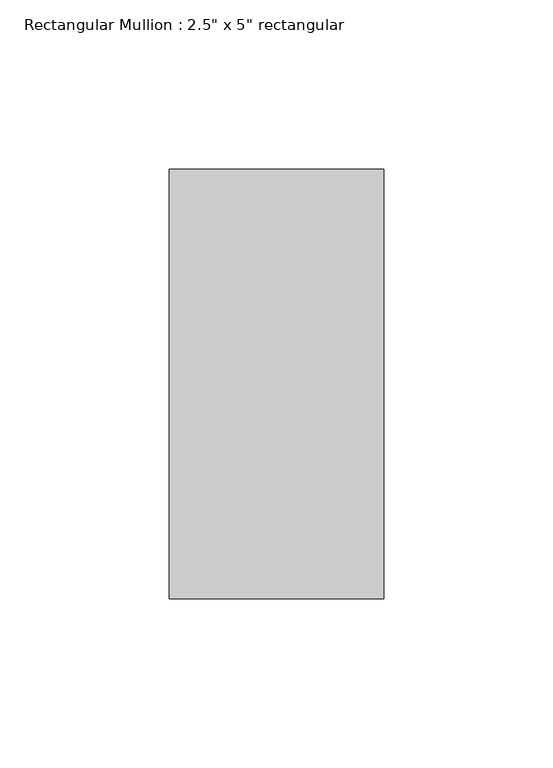
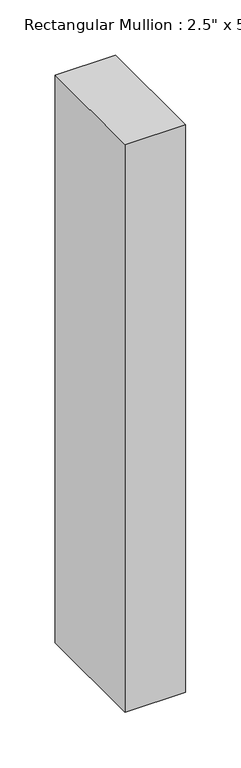
"""IFC4 building model written with IfcOpenShell, lengths in millimetres: member geometry."""

from ifc_helpers import new_model, si_unit, frame, origin, place, context, project, spatial, polyline, outline, extrude, source, transform, mapped, element, save


def member_00d99baf(model_context):
    return source(origin(), model_context, "Body", "SweptSolid", [
        extrude(outline(polyline([(0.0, 63.5), (0.0, -63.5), (-63.5, -63.5), (-63.5, 63.5), (0.0, 63.5)])), frame((0.0, 0.0, -628.65), z_axis=(0.0, 0.0, 1.0), x_axis=(1.0, 0.0, 0.0)), (0.0, 0.0, 1.0), 628.65),
    ])


if __name__ == "__main__":
    model = new_model("IFC4")
    model_context = context("Model", 3, world=origin())
    ifc_project = project(units=[si_unit("LENGTHUNIT", "METRE", prefix="MILLI")], contexts=[model_context])
    site = spatial("IfcSite", under=ifc_project)
    building = spatial("IfcBuilding", under=site)
    placement = place(None, origin())
    member_shape = member_00d99baf(model_context)
    element("IfcMember", 1, ObjectType="Rectangular Mullion : 2.5\" x 5\" rectangular", at=placement, inside=building, context=model_context, shape_type="MappedRepresentation", body=[
        mapped(member_shape, transform((0.0, 0.0, 0.0), x_axis=(1.0, 0.0, 0.0), y_axis=(0.0, 1.0, 0.0), z_axis=(0.0, 0.0, 1.0))),
    ])
    save(model, "model.ifc")

# Revit data of these elements
# Type "Rectangular Mullion : 2.5\" x 5\" rectangular"
#   built-in parameter 1007304 = 0.416667 (stored number, unit not read)
#   built-in parameter 1007301 = 0.104167 (stored number, unit not read)
#   built-in parameter 1007300 = 0.104167 (stored number, unit not read)
# Element 1 (IfcMember, "Rectangular Mullion : 2.5\" x 5\" rectangular")
#   Materials on its faces: "Aluminum"
# Materials
#   "Aluminum": class "Metal", colour RGB 247 247 247, transparency 0, Description = "Aluminum 6061", Cost = 0
